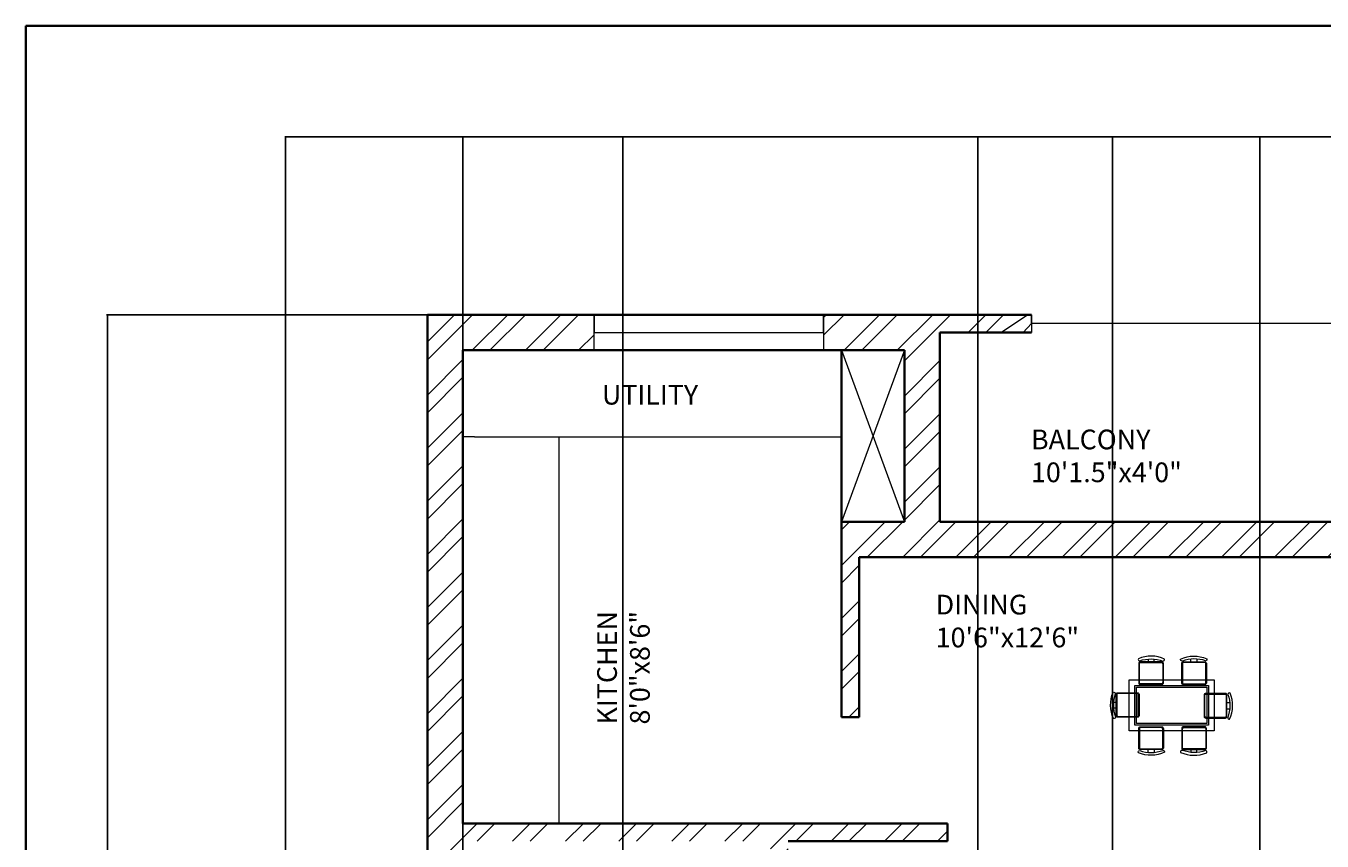
# Model space of a CAD drawing. Units: inches. Extents: x 1513 to 2170, y 1240 to 2288.
# Tile 9 of 10: x 1513 to 1842, y 2081 to 2288. Entities that reach past the tile are written whole.
import ezdxf

# ---------------------------------------------------------------- set-up
doc = ezdxf.new("R2010")
doc.units = ezdxf.units.IN
for name, color, linetype, lineweight in [('A-ANNO-DIMS', 2, 'Continuous', 18), ('A-ANNO-TTLB', 7, 'Continuous', 35), ('A-AREA-IDEN', 7, 'Continuous', 18), ('A-FLOR-FIXT', 9, 'Continuous', 18), ('A-FLOR-HRAL', 7, 'Continuous', 18), ('A-FLOR-OPEN', 7, 'Continuous', 18), ('A-FURN', 8, 'Continuous', 18), ('A-GLAZ', 4, 'Continuous', 18), ('A-WALL', 7, 'Continuous', 35), ('A-WALL-PATT', 252, 'Continuous', 13)]:
    doc.layers.add(name, color=color, linetype=linetype, lineweight=lineweight)
doc.styles.get("Standard").update_dxf_attribs({"font": 'arial.ttf'})
doc.dimstyles.get("Standard").update_dxf_attribs({"dimtxt": 0.18, "dimasz": 0.18, "dimexe": 0.18, "dimexo": 0.0625, "dimgap": 0.09, "dimtad": 0, "dimtih": 1, "dimtoh": 1, "dimdec": 4, "dimzin": 0, "dimdsep": 46, "dimtxsty": 'Standard', "dimcen": 0.09, "dimadec": 0, "dimazin": 0, "dimtfac": 1, "dimtdec": 4, "dimtofl": 0, "dimtmove": 0, "dimatfit": 3, "dimfxl": 1, "dimtolj": 1, "dimtzin": 0, "dimarcsym": 0})

# ---------------------------------------------------------------- blocks, each defined once
blk = doc.blocks.new('TABLE-DINING')
for points in [[(0, 12.94), (21.57, 12.94), (21.57, 0), (0, 0)], [(0, 12.94), (21.57, 12.94), (21.57, 0), (0, 0)], [(1.44, 11.51), (20.13, 11.51), (20.13, 1.44), (1.44, 1.44)], [(1.44, 11.5), (20.13, 11.5), (20.13, 1.44), (1.44, 1.44)], [(1.87, 11.07), (19.7, 11.07), (19.7, 1.87), (1.87, 1.87)], [(1.87, 11.07), (19.7, 11.07), (19.7, 1.87), (1.87, 1.87)]]:
    blk.add_lwpolyline(points, close=True)
blk = doc.blocks.new('CHAIR-DINING-A')
for points in [[(0.35, 6.01, -0.175809), (6.23, 5.97, 0.578392), (6.67, 6.46, 0.214524), (0.04, 6.55, 0.552014), (0.35, 6.01, -0.065079)], [(0.35, 6.01, -0.175809), (6.23, 5.97, 0.578392), (6.67, 6.46, 0.214524), (0.04, 6.55, 0.552014), (0.35, 6.01, -0.065079)], [(5.98, 5.78), (0.53, 5.78, 0.414214), (0.14, 5.4), (0.14, 0.38, 0.414214), (0.53, 0), (5.98, 0, 0.414214), (6.36, 0.38), (6.36, 5.4, 0.414214), (5.98, 5.78)], [(5.98, 5.78), (0.53, 5.78, 0.414214), (0.14, 5.4), (0.14, 0.38, 0.414214), (0.53, 0), (5.98, 0, 0.414214), (6.36, 0.38), (6.36, 5.4, 0.414214), (5.98, 5.78)], [(4.06, 5.78), (4.06, 6.47, -0.064759)], [(4.06, 5.78), (4.06, 6.47, -0.064759)]]:
    blk.add_lwpolyline(points, format="xyb")
blk.add_lwpolyline([(0.53, 5.61), (5.81, 5.61, -0.414214), (6.19, 5.23), (6.19, 0.55, -0.414214), (5.81, 0.17), (0.53, 0.17, -0.512069), (0.32, 0.55), (0.32, 5.23, -0.512069)], format="xyb", close=True)
blk.add_lwpolyline([(0.53, 5.61), (5.81, 5.61, -0.414214), (6.19, 5.23), (6.19, 0.55, -0.414214), (5.81, 0.17), (0.53, 0.17, -0.512069), (0.32, 0.55), (0.32, 5.23, -0.512069)], format="xyb", close=True)
blk.add_lwpolyline([(2.54, 6.48), (2.54, 5.78)])
blk.add_lwpolyline([(2.54, 6.48), (2.54, 5.78)])
blk = doc.blocks.new('CHAIR-DINING-B')
for points in [[(5.98, 1.44), (0.53, 1.44, -0.414214), (0.14, 1.82), (0.14, 6.83, -0.414214), (0.53, 7.22), (5.98, 7.22, -0.414214), (6.36, 6.83), (6.36, 1.82, -0.414214), (5.98, 1.44)], [(5.98, 1.44), (0.53, 1.44, -0.414214), (0.14, 1.82), (0.14, 6.83, -0.414214), (0.53, 7.22), (5.98, 7.22, -0.414214), (6.36, 6.83), (6.36, 1.82, -0.414214), (5.98, 1.44)], [(6.23, 1.25, -0.578392), (6.67, 0.76, -0.214524), (0.04, 0.67, -0.552014), (0.35, 1.2, 0.175809), (6.23, 1.25)], [(6.23, 1.25, -0.578392), (6.67, 0.76, -0.214524), (0.04, 0.67, -0.552014), (0.35, 1.2, 0.175809), (6.23, 1.25)], [(4.06, 1.44), (4.06, 0.75, 0.064759)], [(4.06, 1.44), (4.06, 0.75, 0.064759)]]:
    blk.add_lwpolyline(points, format="xyb")
blk.add_lwpolyline([(0.53, 1.61), (5.81, 1.61, 0.414214), (6.19, 1.99), (6.19, 6.66, 0.414214), (5.81, 7.04), (0.53, 7.04, 0.512069), (0.32, 6.66), (0.32, 1.99, 0.512069)], format="xyb", close=True)
blk.add_lwpolyline([(0.53, 1.61), (5.81, 1.61, 0.414214), (6.19, 1.99), (6.19, 6.66, 0.414214), (5.81, 7.04), (0.53, 7.04, 0.512069), (0.32, 6.66), (0.32, 1.99, 0.512069)], format="xyb", close=True)
blk.add_lwpolyline([(2.54, 0.74), (2.54, 1.44)])
blk.add_lwpolyline([(2.54, 0.74), (2.54, 1.44)])
blk = doc.blocks.new('*D25')
at = {"layer": 'A-ANNO-DIMS', "color": 0, "lineweight": -2, "transparency": 16777216}
for p, q in [((1578.87, 2040.54), (1578.87, 2259.81)), ((1579.05, 2259.63), (1810.07, 2259.63)), ((2041.67, 2259.63), (1810.65, 2259.63)), ((2041.85, 2040.54), (2041.85, 2259.81))]:
    blk.add_line(p, q, dxfattribs=at)
at = {"layer": 'A-ANNO-DIMS', "color": 0, "transparency": 16777216}
for points in [[(1579.05, 2259.66), (1579.05, 2259.6), (1578.87, 2259.63)], [(2041.67, 2259.66), (2041.67, 2259.6), (2041.85, 2259.63)]]:
    blk.add_solid(points, dxfattribs=at)
at = {"layer": 'Defpoints', "color": 0, "transparency": 16777216}
for p in [(2041.85, 2259.63), (1578.87, 2040.48), (2041.85, 2040.48)]:
    blk.add_point(p, dxfattribs=at)
at = {"layer": 'A-ANNO-DIMS', "color": 0, "transparency": 16777216, "insert": (1810.36, 2259.63), "char_height": 0.18, "attachment_point": 5}
blk.add_mtext('\\A1;463', dxfattribs=at)
blk = doc.blocks.new('*D30')
at = {"layer": 'A-ANNO-DIMS', "color": 0, "lineweight": -2, "transparency": 16777216}
for p, q in [((1614.8, 2214.48), (1533.54, 2214.48)), ((1533.72, 2214.3), (1533.72, 2055.66)), ((1533.72, 1896.66), (1533.72, 2055.3)), ((1578.8, 1896.48), (1533.54, 1896.48))]:
    blk.add_line(p, q, dxfattribs=at)
at = {"layer": 'A-ANNO-DIMS', "color": 0, "transparency": 16777216}
for points in [[(1533.69, 2214.3), (1533.75, 2214.3), (1533.72, 2214.48)], [(1533.69, 1896.66), (1533.75, 1896.66), (1533.72, 1896.48)]]:
    blk.add_solid(points, dxfattribs=at)
at = {"layer": 'Defpoints', "color": 0, "transparency": 16777216}
for p in [(1533.72, 2214.48), (1614.87, 2214.48), (1578.87, 1896.48)]:
    blk.add_point(p, dxfattribs=at)
at = {"layer": 'A-ANNO-DIMS', "color": 0, "transparency": 16777216, "insert": (1533.72, 2055.48), "char_height": 0.18, "attachment_point": 5}
blk.add_mtext('\\A1;318', dxfattribs=at)
blk = doc.blocks.new('*D32')
at = {"layer": 'A-ANNO-DIMS', "color": 0, "lineweight": -2, "transparency": 16777216}
for p, q in [((1623.87, 1887.54), (1623.87, 2259.81)), ((1624.05, 2259.63), (1643.84, 2259.63)), ((1664.28, 2259.63), (1644.49, 2259.63)), ((1664.46, 1887.54), (1664.46, 2259.81))]:
    blk.add_line(p, q, dxfattribs=at)
at = {"layer": 'A-ANNO-DIMS', "color": 0, "transparency": 16777216}
for points in [[(1624.05, 2259.66), (1624.05, 2259.6), (1623.87, 2259.63)], [(1664.28, 2259.66), (1664.28, 2259.6), (1664.46, 2259.63)]]:
    blk.add_solid(points, dxfattribs=at)
at = {"layer": 'Defpoints', "color": 0, "transparency": 16777216}
for p in [(1664.46, 2259.63), (1623.87, 1887.48), (1664.46, 1887.48)]:
    blk.add_point(p, dxfattribs=at)
at = {"layer": 'A-ANNO-DIMS', "color": 0, "transparency": 16777216, "insert": (1644.16, 2259.63), "char_height": 0.18, "attachment_point": 5}
blk.add_mtext('\\A1;40.6', dxfattribs=at)
blk = doc.blocks.new('*D33')
at = {"layer": 'A-ANNO-DIMS', "color": 0, "lineweight": -2, "transparency": 16777216}
for p, q in [((1664.46, 1887.54), (1664.46, 2259.81)), ((1664.64, 2259.63), (1709.25, 2259.63)), ((1754.28, 2259.63), (1709.68, 2259.63)), ((1754.46, 1887.54), (1754.46, 2259.81))]:
    blk.add_line(p, q, dxfattribs=at)
at = {"layer": 'A-ANNO-DIMS', "color": 0, "transparency": 16777216}
for points in [[(1664.64, 2259.66), (1664.64, 2259.6), (1664.46, 2259.63)], [(1754.28, 2259.66), (1754.28, 2259.6), (1754.46, 2259.63)]]:
    blk.add_solid(points, dxfattribs=at)
at = {"layer": 'Defpoints', "color": 0, "transparency": 16777216}
for p in [(1754.46, 2259.63), (1664.46, 1887.48), (1754.46, 1887.48)]:
    blk.add_point(p, dxfattribs=at)
at = {"layer": 'A-ANNO-DIMS', "color": 0, "transparency": 16777216, "insert": (1709.46, 2259.63), "char_height": 0.18, "attachment_point": 5}
blk.add_mtext('\\A1;90', dxfattribs=at)
blk = doc.blocks.new('*D37')
at = {"layer": 'A-ANNO-DIMS', "color": 0, "lineweight": -2, "transparency": 16777216}
for p, q in [((1788.59, 1803.54), (1788.59, 2259.81)), ((1788.77, 2259.63), (1806.89, 2259.63)), ((1825.8, 2259.63), (1807.68, 2259.63)), ((1825.98, 1803.54), (1825.98, 2259.81))]:
    blk.add_line(p, q, dxfattribs=at)
at = {"layer": 'A-ANNO-DIMS', "color": 0, "transparency": 16777216}
for points in [[(1788.77, 2259.66), (1788.77, 2259.6), (1788.59, 2259.63)], [(1825.8, 2259.66), (1825.8, 2259.6), (1825.98, 2259.63)]]:
    blk.add_solid(points, dxfattribs=at)
at = {"layer": 'Defpoints', "color": 0, "transparency": 16777216}
for p in [(1825.98, 2259.63), (1788.59, 1803.48), (1825.98, 1803.48)]:
    blk.add_point(p, dxfattribs=at)
at = {"layer": 'A-ANNO-DIMS', "color": 0, "transparency": 16777216, "insert": (1807.28, 2259.63), "char_height": 0.18, "attachment_point": 5}
blk.add_mtext('\\A1;37.39', dxfattribs=at)

msp = doc.modelspace()

# ---------------------------------------------------------------- hatches: boundary and pattern name
at = {"layer": 'A-WALL-PATT'}
h = msp.add_hatch(dxfattribs=at)
h.set_pattern_fill('ANSI32', color=256)
h.paths.add_polyline_path([(2041.852, 1719.48), (2014.852, 1719.48), (2014.852, 1734.444), (2005.852, 1734.444), (2005.852, 1710.48), (2032.852, 1710.48), (2032.852, 1663.98), (1976.619, 1663.98), (1976.619, 1659.48), (2005.852, 1659.48), (2005.852, 1626.27), (2014.852, 1626.27), (2014.852, 1659.48), (2041.852, 1659.48)])
h.paths.add_polyline_path([(1954.521, 1663.98), (1875.357, 1663.98), (1875.357, 1659.48), (1945.852, 1659.48), (1945.852, 1546.98), (1950.352, 1546.98), (2005.852, 1546.98), (2005.852, 1422.48), (1985.47, 1422.48), (1985.47, 1413.48), (2014.852, 1413.48), (2014.852, 1602.27), (2005.852, 1602.27), (2005.852, 1551.48), (1950.352, 1551.48), (1950.352, 1659.48), (1954.521, 1659.48)])
h.paths.add_polyline_path([(1949.47, 1422.48), (1937.366, 1422.48), (1937.366, 1413.48), (1949.47, 1413.48)], flags=0)
h.paths.add_polyline_path([(1937.366, 1422.48), (1908.866, 1422.48), (1908.866, 1546.98), (1805.486, 1546.98), (1805.486, 1542.48), (1904.366, 1542.48), (1904.366, 1451.2), (1897.222, 1451.2), (1897.222, 1442.2), (1904.366, 1442.2), (1904.366, 1422.48), (1904.366, 1413.48), (1904.366, 1389.48), (1908.866, 1389.48), (1908.866, 1413.48), (1932.866, 1413.48), (1932.866, 1389.48), (1937.366, 1389.48)])
h.paths.add_polyline_path([(1830.254, 1442.2), (1844.144, 1442.2), (1844.144, 1451.2), (1830.254, 1451.2), (1821.254, 1451.2), (1821.254, 1422.48), (1766.366, 1422.48), (1766.366, 1542.48), (1770.265, 1542.48), (1770.265, 1546.98), (1758.774, 1546.98), (1758.774, 1544.73), (1758.774, 1542.48), (1761.866, 1542.48), (1761.866, 1389.48), (1779.454, 1389.48), (1779.454, 1398.48), (1770.866, 1398.48), (1770.866, 1413.48), (1830.254, 1413.48)])
h.paths.add_polyline_path([(1686.156, 1451.2), (1677.156, 1451.2), (1677.156, 1422.48), (1623.866, 1422.48), (1623.866, 1460.073), (1614.866, 1460.073), (1614.866, 1413.48), (1686.156, 1413.48)])
h.paths.add_polyline_path([(1761.866, 1422.48), (1686.156, 1422.48), (1686.156, 1413.48), (1761.866, 1413.48)])
h.paths.add_polyline_path([(1623.866, 1542.48), (1688.266, 1542.48), (1688.266, 1544.73), (1688.266, 1546.98), (1623.866, 1546.98), (1623.866, 1560.442), (1614.866, 1560.442), (1614.866, 1520.073), (1619.366, 1520.073), (1623.866, 1520.073)])
h.paths.add_polyline_path([(1623.866, 1600.98), (1715.366, 1600.98), (1715.366, 1546.98), (1711.055, 1546.98), (1711.055, 1542.48), (1719.866, 1542.48), (1726.867, 1542.48), (1726.867, 1544.73), (1726.867, 1546.98), (1719.866, 1546.98), (1719.866, 1600.98), (1719.866, 1608.301), (1717.616, 1608.301), (1715.366, 1608.301), (1715.366, 1605.48), (1623.866, 1605.48), (1623.866, 1620.254), (1614.866, 1620.254), (1614.866, 1584.442), (1623.866, 1584.442)])
h.paths.add_polyline_path([(1623.866, 1659.48), (1715.366, 1659.48), (1715.366, 1629.2), (1719.866, 1629.2), (1719.866, 1659.48), (1767.866, 1659.48), (1767.866, 1629.2), (1772.366, 1629.2), (1772.366, 1663.98), (1578.866, 1663.98), (1578.866, 1661.73), (1578.866, 1659.48), (1578.866, 1635.48), (1583.366, 1635.48), (1583.366, 1654.98), (1614.866, 1654.98), (1614.866, 1644.254), (1619.366, 1644.254), (1623.866, 1644.254)])
h.paths.add_polyline_path([(1788.587, 1798.98), (1788.587, 1803.48), (1623.866, 1803.48), (1623.866, 1887.48), (1829.49, 1887.48), (1829.49, 1891.98), (1829.49, 1896.48), (1748.366, 1896.48), (1743.866, 1896.48), (1623.866, 1896.48), (1623.866, 1904.333), (1619.366, 1904.333), (1614.866, 1904.333), (1614.866, 1896.48), (1578.866, 1896.48), (1578.866, 1887.48), (1614.866, 1887.48), (1614.866, 1803.48), (1578.866, 1803.48), (1578.866, 1794.48), (1626.866, 1794.48), (1788.587, 1794.48)])
h.paths.add_polyline_path([(1635.866, 1794.48), (1626.866, 1794.48), (1626.866, 1763.627), (1631.366, 1763.627), (1635.866, 1763.627)])
h.paths.add_polyline_path([(1635.866, 1703.627), (1626.866, 1703.627), (1626.866, 1663.98), (1635.866, 1663.98)])
h.paths.add_polyline_path([(1587.866, 2016.48), (1614.866, 2016.48), (1623.866, 2016.48), (1707.767, 2016.48), (1707.767, 2018.73), (1707.767, 2020.98), (1706.366, 2020.98), (1706.366, 2025.944), (1701.866, 2025.944), (1701.866, 2020.98), (1623.866, 2020.98), (1623.866, 2045.903), (1614.866, 2045.903), (1614.866, 2025.48), (1583.366, 2025.48), (1583.366, 2040.48), (1578.866, 2040.48), (1578.866, 2016.48), (1578.866, 1956.48), (1614.866, 1956.48), (1614.866, 1946.333), (1623.866, 1946.333), (1623.866, 1965.48), (1587.866, 1965.48)])
h.paths.add_polyline_path([(1748.366, 2016.48), (1748.366, 2025.48), (1743.866, 2025.48), (1739.366, 2025.48), (1739.366, 2020.98), (1738.09, 2020.98), (1738.09, 2016.48), (1743.866, 2016.48), (1743.866, 1896.48), (1748.366, 1896.48)])
h.paths.add_polyline_path([(1746.736, 2085.48), (1623.866, 2085.48), (1623.866, 2205.48), (1657.136, 2205.48), (1657.136, 2214.48), (1614.866, 2214.48), (1614.866, 2069.903), (1623.866, 2069.903), (1623.866, 2080.98), (1683.866, 2080.98), (1701.866, 2080.98), (1701.866, 2046.743), (1706.366, 2046.743), (1706.366, 2080.98), (1746.736, 2080.98)])
h = msp.add_hatch(dxfattribs=at)
h.set_pattern_fill('ANSI32', color=256)
h.paths.add_polyline_path([(1744.852, 2209.98), (1762.042, 2209.98), (1762.042, 2214.48), (1715.345, 2214.48), (1715.345, 2205.48), (1735.852, 2205.48), (1735.852, 2161.98), (1733.253, 2161.98), (1719.866, 2161.98), (1719.866, 2112.429), (1724.366, 2112.429), (1724.366, 2152.98), (1762.042, 2152.98), (1870.852, 2152.98), (1870.852, 2080.98), (1875.352, 2080.98), (1878.245, 2080.98), (1878.245, 2083.23), (1878.245, 2085.48), (1875.352, 2085.48), (1875.352, 2173.929), (1881.628, 2173.929), (1881.628, 2178.429), (1881.628, 2182.929), (1875.352, 2182.929), (1875.352, 2214.48), (1858.335, 2214.48), (1858.335, 2209.98), (1866.352, 2209.98), (1866.352, 2161.98), (1762.042, 2161.98), (1744.852, 2161.98)])
h.paths.add_polyline_path([(2014.852, 2214.48), (1944.011, 2214.48), (1944.011, 2182.929), (1938.347, 2182.929), (1938.347, 2173.929), (1953.011, 2173.929), (1953.011, 2182.929), (1953.011, 2205.48), (2005.852, 2205.48), (2005.852, 2085.48), (1955.061, 2085.48), (1955.061, 2080.98), (2005.852, 2080.98), (2005.852, 2068.903), (2014.852, 2068.903)])
h.paths.add_polyline_path([(2014.852, 2044.903), (2005.852, 2044.903), (2005.852, 2020.98), (1926.352, 2020.98), (1926.352, 2080.98), (1930.882, 2080.98), (1930.882, 2083.23), (1930.882, 2085.48), (1921.852, 2085.48), (1915.536, 2085.48), (1915.536, 2083.23), (1915.536, 2080.98), (1921.852, 2080.98), (1921.852, 2020.98), (1916.378, 2020.98), (1916.378, 2018.73), (1916.378, 2016.48), (2005.852, 2016.48), (2005.852, 2009.442), (2014.852, 2009.442), (2014.852, 2016.48), (2029.852, 2016.48), (2041.852, 2016.48), (2041.852, 2040.48), (2037.352, 2040.48), (2037.352, 2036.595), (2037.352, 2020.98), (2014.852, 2020.98)])
h.paths.add_polyline_path([(2041.852, 1956.48), (2014.852, 1956.48), (2014.852, 1963.797), (2005.852, 1963.797), (2005.852, 1947.48), (2032.852, 1947.48), (2032.852, 1896.48), (1978.852, 1896.48), (1978.852, 1891.98), (1978.852, 1887.48), (2005.852, 1887.48), (2005.852, 1862.401), (2014.852, 1862.401), (2014.852, 1887.48), (2037.352, 1887.48), (2037.352, 1863.48), (2041.852, 1863.48), (2041.852, 1887.48), (2041.852, 1896.48)], flags=17)
h.paths.add_polyline_path([(1885.852, 1896.48), (1885.852, 1920.48), (1878.866, 1920.48), (1878.866, 2016.48), (1881.925, 2016.48), (1881.925, 2018.73), (1881.925, 2020.98), (1874.366, 2020.98), (1874.366, 1896.48), (1864.508, 1896.48), (1864.508, 1887.48), (1876.852, 1887.48), (1876.852, 1855.773), (1885.852, 1855.773), (1885.852, 1868.947), (1942.852, 1868.947), (1942.852, 1803.48), (1885.852, 1803.48), (1885.852, 1817.861), (1876.852, 1817.861), (1876.852, 1803.48), (1825.976, 1803.48), (1825.976, 1798.98), (1825.976, 1794.48), (1832.366, 1794.48), (1832.366, 1663.98), (1832.366, 1659.48), (1841.939, 1659.48), (1841.939, 1661.73), (1841.939, 1663.98), (1836.866, 1663.98), (1836.866, 1794.48), (1992.866, 1794.48), (2005.852, 1794.48), (2005.852, 1784.304), (2010.352, 1784.304), (2014.852, 1784.304), (2014.852, 1794.48), (2041.852, 1794.48), (2041.852, 1803.48), (2014.852, 1803.48), (2014.852, 1838.401), (2005.852, 1838.401), (2005.852, 1803.48), (1951.852, 1803.48), (1951.852, 1887.48), (1956.114, 1887.48), (1956.114, 1891.98), (1956.114, 1896.48), (1951.852, 1896.48), (1951.852, 1920.48), (1947.352, 1920.48), (1947.352, 1896.48), (1942.852, 1896.48), (1942.852, 1877.947), (1885.852, 1877.947)])

# ---------------------------------------------------------------- linework, layer by layer
at = {"layer": 'A-ANNO-TTLB'}
msp.add_lwpolyline([(1513.071, 2287.731), (2170.435, 2287.731), (2170.435, 1239.669), (1513.071, 1239.669)], close=True, dxfattribs=at)
at = {"layer": 'A-FLOR-FIXT'}
for p, q in [((1626.86, 2183.531), (1623.866, 2183.531)), ((1626.86, 2183.531), (1719.866, 2183.531)), ((1648.301, 2085.48), (1648.301, 2183.531))]:
    msp.add_line(p, q, dxfattribs=at)
at = {"layer": 'A-FLOR-HRAL'}
for p, q in [((1768.065, 2212.23), (1768.065, 2214.48)), ((1768.065, 2214.48), (1768.065, 2209.98)), ((1858.335, 2212.23), (1768.065, 2212.23))]:
    msp.add_line(p, q, dxfattribs=at)
at = {"layer": 'A-FLOR-OPEN'}
for p, q in [((1719.866, 2205.48), (1735.852, 2161.98)), ((1735.852, 2205.48), (1719.866, 2161.98))]:
    msp.add_line(p, q, dxfattribs=at)
at = {"layer": 'A-FURN'}
for points in [[(1789.359, 2112.508, -0.5783921), (1788.87, 2112.063, -0.2145244), (1788.781, 2118.694, -0.552014), (1789.315, 2118.383, 0.1758094), (1789.359, 2112.508)], [(1789.359, 2112.508, -0.5783921), (1788.87, 2112.063, -0.2145244), (1788.781, 2118.694, -0.552014), (1789.315, 2118.383, 0.1758094), (1789.359, 2112.508)], [(1789.55, 2118.211, -0.4142136), (1789.932, 2118.593), (1794.946, 2118.593, -0.4142136), (1795.328, 2118.211), (1795.328, 2112.758, -0.4142136), (1794.946, 2112.376), (1789.932, 2112.376, -0.4142136), (1789.55, 2112.758), (1789.55, 2118.211)], [(1789.55, 2118.211, -0.4142136), (1789.932, 2118.593), (1794.947, 2118.593, -0.4142136), (1795.328, 2118.211), (1795.328, 2112.757, -0.4142136), (1794.947, 2112.376), (1789.932, 2112.376, -0.4142136), (1789.55, 2112.757), (1789.55, 2118.211)], [(1817.635, 2118.025, 0.4142136), (1817.253, 2118.406), (1812.238, 2118.406, 0.4142136), (1811.857, 2118.025), (1811.857, 2112.571, 0.4142136), (1812.238, 2112.189), (1817.253, 2112.189, 0.4142136), (1817.635, 2112.571), (1817.635, 2118.025)], [(1817.635, 2118.024, 0.4142136), (1817.253, 2118.406), (1812.238, 2118.406, 0.4142136), (1811.857, 2118.024), (1811.857, 2112.571, 0.4142136), (1812.238, 2112.189), (1817.253, 2112.189, 0.4142136), (1817.635, 2112.571), (1817.635, 2118.024)], [(1817.87, 2118.196, -0.1758092), (1817.826, 2112.322, 0.5783921), (1818.315, 2111.876, 0.2145244), (1818.404, 2118.508, 0.552014), (1817.87, 2118.196, -0.065079)], [(1817.87, 2118.196, -0.1758092), (1817.826, 2112.321, 0.5783921), (1818.315, 2111.876, 0.2145244), (1818.404, 2118.507, 0.552014), (1817.87, 2118.196, -0.065079)], [(1789.55, 2114.673), (1788.861, 2114.673, 0.0647586)], [(1789.55, 2114.673), (1788.861, 2114.673, 0.0647586)], [(1817.635, 2114.486), (1818.324, 2114.486, -0.0647586)], [(1817.635, 2114.486), (1818.324, 2114.486, -0.0647586)], [(1812.028, 2104.168, 0.4142136), (1812.41, 2104.549), (1812.41, 2109.564, 0.4142136), (1812.028, 2109.945), (1806.574, 2109.945, 0.4142136), (1806.193, 2109.564), (1806.193, 2104.549, 0.4142136), (1806.574, 2104.168), (1812.028, 2104.168)], [(1812.028, 2104.167, 0.4142136), (1812.41, 2104.549), (1812.41, 2109.563, 0.4142136), (1812.028, 2109.945), (1806.574, 2109.945, 0.4142136), (1806.193, 2109.563), (1806.193, 2104.549, 0.4142136), (1806.574, 2104.167), (1812.028, 2104.167)], [(1812.2, 2103.932, -0.1758093), (1806.325, 2103.976, 0.5783921), (1805.88, 2103.487, 0.2145244), (1812.511, 2103.398, 0.552014), (1812.2, 2103.932, -0.065079)], [(1812.2, 2103.932, -0.1758093), (1806.325, 2103.976, 0.5783921), (1805.88, 2103.487, 0.2145244), (1812.511, 2103.398, 0.552014), (1812.2, 2103.932, -0.065079)], [(1808.49, 2104.168), (1808.49, 2103.478, -0.0647586)], [(1808.49, 2104.167), (1808.49, 2103.478, -0.0647586)]]:
    msp.add_lwpolyline(points, format="xyb", dxfattribs=at)
for points in [[(1789.722, 2118.209), (1789.722, 2112.929, 0.4142136), (1790.104, 2112.548), (1794.775, 2112.548, 0.4142136), (1795.156, 2112.929), (1795.156, 2118.209, 0.5120695), (1794.775, 2118.421), (1790.104, 2118.421, 0.5120695)], [(1789.722, 2118.209), (1789.722, 2112.929, 0.4142136), (1790.104, 2112.548), (1794.775, 2112.548, 0.4142136), (1795.156, 2112.929), (1795.156, 2118.209, 0.5120695), (1794.775, 2118.421), (1790.104, 2118.421, 0.5120695)], [(1817.463, 2118.022), (1817.463, 2112.743, -0.4142136), (1817.081, 2112.361), (1812.41, 2112.361, -0.4142136), (1812.029, 2112.743), (1812.029, 2118.022, -0.5120695), (1812.41, 2118.234), (1817.081, 2118.234, -0.5120695)], [(1817.463, 2118.022), (1817.463, 2112.742, -0.4142136), (1817.081, 2112.361), (1812.41, 2112.361, -0.4142136), (1812.029, 2112.742), (1812.029, 2118.022, -0.5120695), (1812.41, 2118.234), (1817.081, 2118.234, -0.5120695)], [(1812.026, 2104.339), (1806.746, 2104.339, -0.4142136), (1806.365, 2104.721), (1806.365, 2109.392, -0.4142136), (1806.746, 2109.773), (1812.026, 2109.773, -0.5120695), (1812.238, 2109.392), (1812.238, 2104.721, -0.5120695)], [(1812.026, 2104.339), (1806.746, 2104.339, -0.4142136), (1806.365, 2104.721), (1806.365, 2109.392, -0.4142136), (1806.746, 2109.773), (1812.026, 2109.773, -0.5120695), (1812.238, 2109.392), (1812.238, 2104.721, -0.5120695)]]:
    msp.add_lwpolyline(points, format="xyb", close=True, dxfattribs=at)
for points in [[(1788.848, 2116.2), (1789.55, 2116.2)], [(1788.848, 2116.2), (1789.55, 2116.2)], [(1818.337, 2116.013), (1817.635, 2116.013)], [(1818.337, 2116.013), (1817.635, 2116.013)], [(1810.017, 2103.465), (1810.017, 2104.168)], [(1810.017, 2103.465), (1810.017, 2104.167)]]:
    msp.add_lwpolyline(points, dxfattribs=at)
at = {"layer": 'A-GLAZ'}
for p, q in [((1657.136, 2205.48), (1657.136, 2214.48)), ((1657.136, 2214.48), (1657.136, 2209.98)), ((1715.345, 2209.98), (1715.345, 2214.48)), ((1715.345, 2214.48), (1715.345, 2205.48)), ((1657.136, 2209.98), (1693.136, 2209.98)), ((1693.136, 2209.98), (1715.345, 2209.98))]:
    msp.add_line(p, q, dxfattribs=at)
at = {"layer": 'A-WALL'}
for p, q in [((1614.866, 2214.48), (1768.065, 2214.48)), ((1614.866, 2214.48), (1614.866, 2025.48)), ((1762.042, 2209.98), (1744.852, 2209.98)), ((1744.852, 2209.98), (1744.852, 2161.98)), ((1762.042, 2209.98), (1768.065, 2209.98)), ((1623.866, 2205.48), (1735.852, 2205.48)), ((1623.866, 2205.48), (1623.866, 2085.48)), ((1719.866, 2205.48), (1719.866, 2112.429)), ((1735.852, 2161.98), (1735.852, 2205.48)), ((1735.852, 2161.98), (1719.866, 2161.98)), ((1735.852, 2161.98), (1733.253, 2161.98)), ((1762.042, 2161.98), (1744.852, 2161.98)), ((1762.042, 2161.98), (1866.352, 2161.98)), ((1724.366, 2152.98), (1762.042, 2152.98)), ((1724.366, 2152.98), (1724.366, 2112.429)), ((1762.042, 2152.98), (1870.852, 2152.98)), ((1724.366, 2112.429), (1719.866, 2112.429)), ((1623.866, 2085.48), (1746.736, 2085.48)), ((1746.736, 2080.98), (1746.736, 2085.48)), ((1706.366, 2080.98), (1746.736, 2080.98))]:
    msp.add_line(p, q, dxfattribs=at)
at = {"layer": 'A-WALL-PATT'}
for p, q in [((1760.266, 2209.98), (1767.091, 2214.48)), ((1765.972, 2209.98), (1768.065, 2212.23))]:
    msp.add_line(p, q, dxfattribs=at)

# ---------------------------------------------------------------- block references
at = {"layer": 'A-FURN'}
for name, p in [('CHAIR-DINING-A', (1795.15, 2120.68)), ('TABLE-DINING', (1792.84, 2108.91)), ('CHAIR-DINING-B', (1795.15, 2102.73))]:
    msp.add_blockref(name, p, dxfattribs=at)
at = {"layer": 'A-FURN', "extrusion": (0, 0, -1), "zscale": -1}
msp.add_blockref('CHAIR-DINING-A', (-1812.555, 2120.68), dxfattribs=at)

# ---------------------------------------------------------------- texts
at = {"layer": 'A-AREA-IDEN', "char_height": 5, "attachment_point": 1}
for s, width, insert in [('UTILITY', 90.72073, (1659.12, 2196.697)), ('BALCONY\\P10\'1.5"x4\'0"', 136.63903, (1767.936, 2185.344)), ('DINING\\P10\'6"x12\'6"', 139.6185, (1743.768, 2143.454))]:
    msp.add_mtext_dynamic_manual_height_columns(s, width=width, gutter_width=12.5, heights=[0], dxfattribs=dict(at, insert=insert))
at = {"layer": 'A-AREA-IDEN', "insert": (1657.932, 2110.554), "char_height": 5, "attachment_point": 1, "rotation": 90}
msp.add_mtext_dynamic_manual_height_columns('KITCHEN\\P8\'0"x8\'6"', width=117.57161, gutter_width=12.5, heights=[0], dxfattribs=at)

# ---------------------------------------------------------------- dimensions: what is measured, and where the dimension line sits
at = {"layer": 'A-ANNO-DIMS'}
for base, p1, p2, override, picture, middle in [((2041.852, 2259.63), (1578.866, 2040.48), (2041.852, 2040.48), {"dimdec": 0, "dimlfac": 1, "dimrnd": 0, "dimzin": 0, "dimdsep": 46, "dimlunit": 2}, '*D25', (1810.359, 2259.63)), ((1664.464, 2259.63), (1623.866, 1887.48), (1664.464, 1887.48), {"dimdec": 1, "dimlfac": 1, "dimrnd": 0, "dimzin": 0, "dimdsep": 46, "dimlunit": 2}, '*D32', (1644.165, 2259.63)), ((1754.464, 2259.63), (1664.464, 1887.48), (1754.464, 1887.48), {"dimdec": 0, "dimlfac": 1, "dimrnd": 0, "dimzin": 0, "dimdsep": 46, "dimlunit": 2}, '*D33', (1709.464, 2259.63)), ((1825.976, 2259.63), (1788.587, 1803.48), (1825.976, 1803.48), {"dimdec": 2, "dimlfac": 1, "dimrnd": 0, "dimzin": 0, "dimdsep": 46, "dimlunit": 2}, '*D37', (1807.281, 2259.63))]:
    dim = msp.add_linear_dim(base=base, p1=p1, p2=p2, dimstyle='Standard', override=override, dxfattribs=at)
    dim.commit()
    dim.dimension.update_dxf_attribs({"geometry": picture, "text_midpoint": middle})
dim = msp.add_linear_dim(base=(1533.716, 2214.48), p1=(1578.866, 1896.48), p2=(1614.866, 2214.48), angle=90, dimstyle='Standard', override={"dimdec": 0, "dimlfac": 1, "dimrnd": 0, "dimzin": 0, "dimdsep": 46, "dimlunit": 2}, dxfattribs=at)
dim.commit()
dim.dimension.update_dxf_attribs({"geometry": '*D30', "text_midpoint": (1533.716, 2055.48)})

doc.saveas('drawing.dxf')
